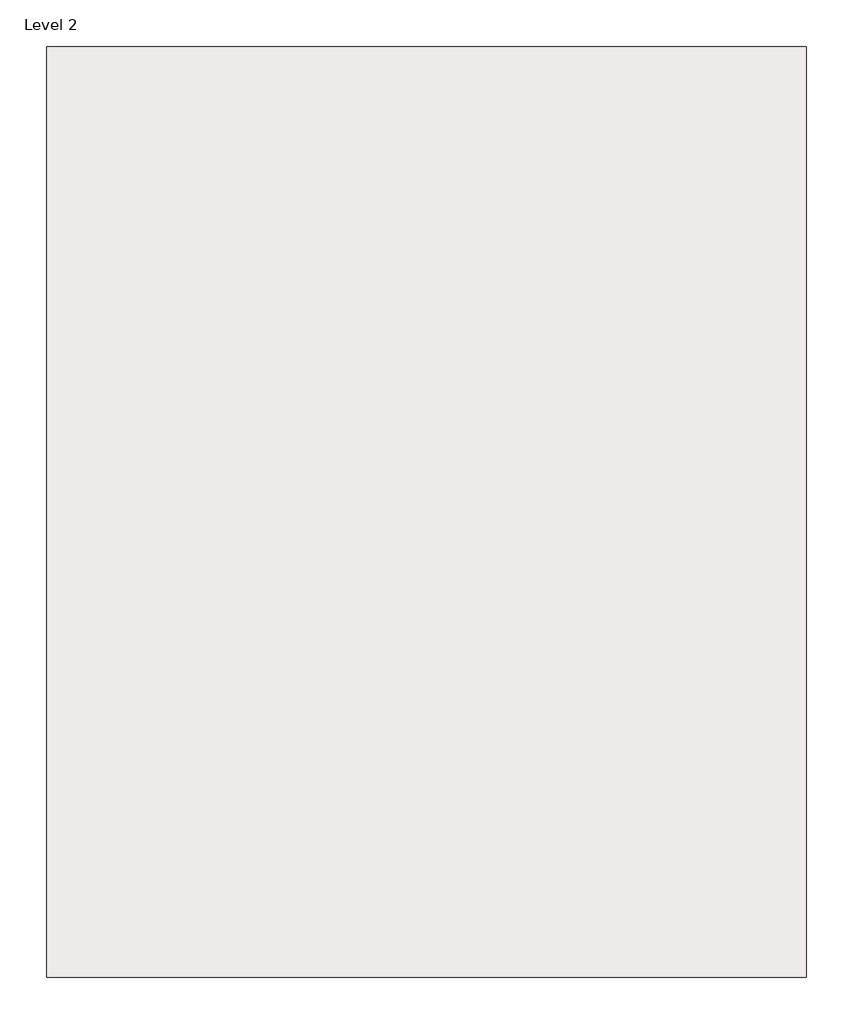
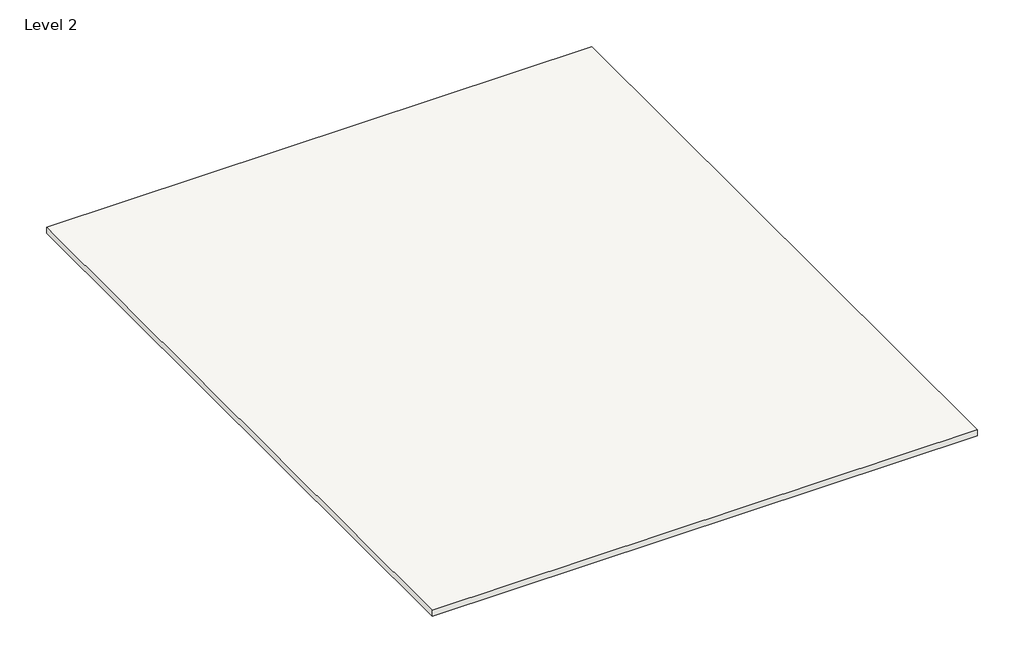
# One storey: 1 roof.
"""IFC4 building model written with IfcOpenShell, lengths in millimetres."""

from ifc_helpers import new_model, si_unit, frame, origin, place, context, project, spatial, polyline, outline, extrude, element, save

model = new_model("IFC4")

# Units and contexts
model_context = context("Model", 3, world=origin())
ifc_project = project(units=[si_unit("LENGTHUNIT", "METRE", prefix="MILLI")], contexts=[model_context])

# Site, building, storey
site = spatial("IfcSite", under=ifc_project)
building = spatial("IfcBuilding", under=site)
storey = spatial("IfcBuildingStorey", under=building, Name="Level 2", Elevation=3048.0)

# Roof
placement = place(None, origin())
element("IfcRoof", 1, ObjectType="Generic - 12\"", at=placement, inside=storey, context=model_context, shape_type="SweptSolid", body=[
    extrude(outline(polyline([(-7919.6243007, 9691.577558), (5262.9756993, 9691.577558), (5262.9756993, -6462.822442), (-7919.6243007, -6462.822442), (-7919.6243007, 9691.577558)])), frame((0.0, 0.0, 3048.0), z_axis=(0.0, 0.0, 1.0), x_axis=(1.0, 0.0, 0.0)), (0.0, 0.0, 1.0), 152.4),
])

save(model, "model.ifc")

# Revit data of these elements
# Type "Generic - 12\""
#   Assembly Code = "B1020"
#   Layers, outside or top first: 0' - 6" no material (function 1)
# Element 1 (IfcRoof, "Generic - 12\"")
#   built-in parameter 1001705 = 10.5 (stored number, unit not read)
#   built-in parameter 1001710 = 33615
#   Phase Created = New Construction
#   Materials on its faces: "Default Roof"
# Materials
#   "Default Roof": colour RGB 88 101 114, transparency 0, Cost = 0
